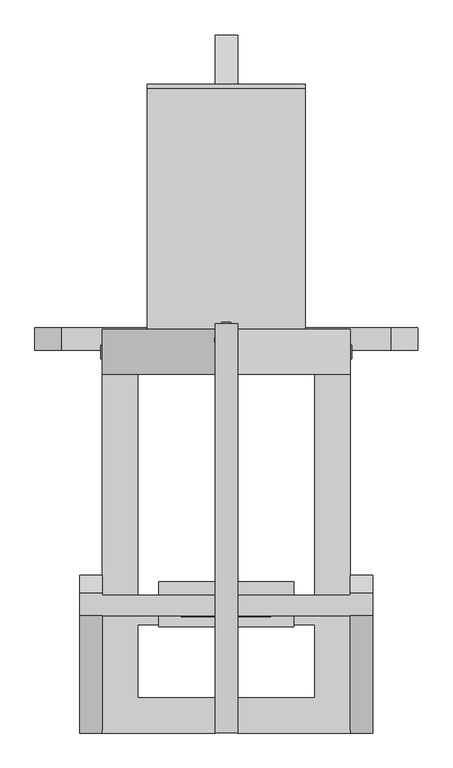
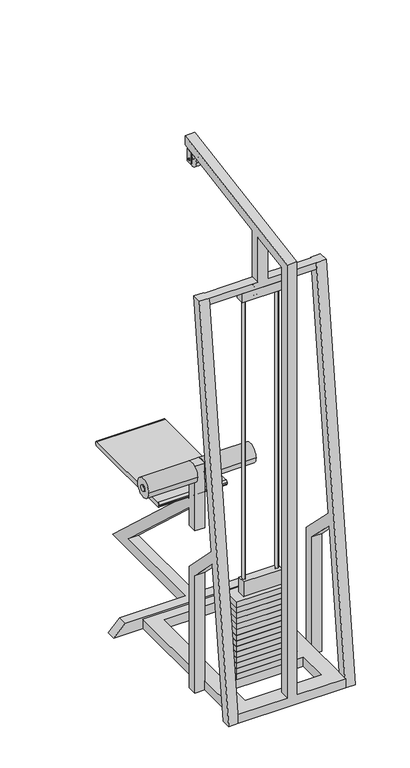
"""IFC4 building model written with IfcOpenShell, lengths in millimetres: proxy geometry."""

from ifc_helpers import new_model, si_unit, point, frame, frame_2d, origin, place, context, project, spatial, polyline, circle_curve, trimmed, segment, composite_curve, outline, extrude, faceted_brep, source, transform, mapped, element, save


def specialty_equipment_45cd0696(model_context):
    return source(origin(), model_context, "Body", "SolidModel", [
        faceted_brep([(130.0819672, 609.7754547, 50.0), (130.0819672, 609.7754547, 0.0), (130.0819672, 109.7754547, 0.0), (130.0819672, 109.7754547, 50.0), (130.0819672, -240.2245453, 0.0), (130.0819672, -240.2245453, 50.0), (130.0819672, -234.1780337, 50.0), (130.0819672, 59.7754547, 0.0), (130.0819672, -189.8602693, 0.0), (130.0819672, -183.8137577, 50.0), (130.0819672, 59.7754547, 50.0), (680.0819672, 609.7754547, 0.0), (680.0819672, 609.7754547, 50.0), (680.0819672, 109.7754547, 50.0), (680.0819672, 109.7754547, 0.0), (680.0819672, -240.2245453, 50.0), (680.0819672, -240.2245453, 0.0), (680.0819672, -234.1780337, 50.0), (680.0819672, 59.7754547, 50.0), (680.0819672, -183.8137577, 50.0), (680.0819672, -189.8602693, 0.0), (680.0819672, 59.7754547, 0.0), (380.0819672, -240.2245453, 50.0), (380.0819672, -190.2245453, 50.0), (430.0819672, -190.2245453, 50.0), (430.0819672, -240.2245453, 50.0), (210.0819672, 559.7754547, 50.0), (600.0819672, 559.7754547, 50.0), (600.0819672, 49.7754547, 50.0), (210.0819672, 49.7754547, 50.0), (210.0819672, -0.2245453, 50.0), (600.0819672, -0.2245453, 50.0), (600.0819672, -160.2245453, 50.0), (210.0819672, -160.2245453, 50.0), (730.0819672, 109.7754547, 0.0), (730.0819672, 59.7754547, 0.0), (730.0819672, -189.8602693, 0.0), (730.0819672, -240.2245453, 0.0), (80.0819672, -240.2245453, 0.0), (80.0819672, -189.8602693, 0.0), (80.0819672, 59.7754547, 0.0), (80.0819672, 109.7754547, 0.0), (600.0819672, 559.7754547, 0.0), (210.0819672, 559.7754547, 0.0), (210.0819672, 49.7754547, 0.0), (600.0819672, 49.7754547, 0.0), (600.0819672, -0.2245453, 0.0), (210.0819672, -0.2245453, 0.0), (210.0819672, -160.2245453, 0.0), (600.0819672, -160.2245453, 0.0), (430.0819672, -240.2245453, 2400.0), (380.0819672, -240.2245453, 2400.0), (380.0819672, 667.995404, 2551.3699916), (380.0819672, 667.995404, 2500.6803038), (380.0819672, 70.1397307, 2401.0376916), (380.0819672, 70.1397307, 2150.0), (380.0819672, 65.9071726, 2150.0), (380.0819672, 19.7754547, 2150.0), (380.0819672, 19.7754547, 2392.6436456), (380.0819672, -190.2245453, 2357.6436456), (430.0819672, -190.2245453, 2357.6436456), (430.0819672, 19.7754547, 2392.6436456), (430.0819672, 19.7754547, 2150.0), (430.0819672, 65.9071726, 2150.0), (430.0819672, 70.1397307, 2150.0), (430.0819672, 70.1397307, 2401.0376916), (430.0819672, 667.995404, 2500.6803038), (430.0819672, 667.995404, 2551.3699916), (130.0819672, 19.7754547, 2150.0), (130.0819672, 19.7754547, 2115.0), (680.0819672, 19.7754547, 2115.0), (680.0819672, 19.7754547, 2150.0), (130.0819672, 65.9071726, 2150.0), (130.0819672, 70.1397307, 2150.0), (80.0819672, 70.1397307, 2150.0), (80.0819672, 19.7754547, 2150.0), (730.0819672, 19.7754547, 2150.0), (730.0819672, 70.1397307, 2150.0), (680.0819672, 70.1397307, 2150.0), (680.0819672, 65.9071726, 2150.0), (680.0819672, 65.9071726, 2115.0), (130.0819672, 65.9071726, 2115.0), (730.0819672, -94.0850882, 791.9870741), (730.0819672, 59.7754547, 638.1265312), (730.0819672, 109.7754547, 658.8372093), (730.0819672, -86.4565503, 855.0692143), (680.0819672, -86.4565503, 855.0692143), (680.0819672, 109.7754547, 658.8372093), (680.0819672, 59.7754547, 638.1265312), (680.0819672, -94.0850882, 791.9870741), (80.0819672, -86.4565503, 855.0692143), (80.0819672, 109.7754547, 658.8372093), (80.0819672, 59.7754547, 638.1265312), (80.0819672, -94.0850882, 791.9870741), (130.0819672, -94.0850882, 791.9870741), (130.0819672, 59.7754547, 638.1265312), (130.0819672, 109.7754547, 658.8372093), (130.0819672, -86.4565503, 855.0692143)], [[[0, 1, 2, 3]], [[4, 5, 6]], [[7, 8, 9, 10]], [[11, 12, 13, 14]], [[15, 16, 17]], [[18, 19, 20, 21]], [[12, 0, 3, 10, 9, 6, 5, 22, 23, 24, 25, 15, 17, 19, 18, 13], [26, 27, 28, 29], [30, 31, 32, 33]], [[1, 0, 12, 11]], [[1, 11, 14, 34, 35, 21, 20, 36, 37, 16, 4, 38, 39, 8, 7, 40, 41, 2], [42, 43, 44, 45], [46, 47, 48, 49]], [[42, 27, 26, 43]], [[27, 42, 45, 28]], [[31, 46, 49, 32]], [[16, 15, 25, 50, 51, 22, 5, 4]], [[43, 26, 29, 44]], [[47, 30, 33, 48]], [[45, 44, 29, 28]], [[47, 46, 31, 30]], [[49, 48, 33, 32]], [[51, 52, 53, 54, 55, 56, 57, 58, 59, 23, 22]], [[60, 61, 62, 63, 64, 65, 66, 67, 50, 25, 24]], [[52, 51, 50, 67]], [[53, 52, 67, 66]], [[59, 58, 61, 60]], [[59, 60, 24, 23]], [[54, 53, 66, 65]], [[55, 54, 65, 64]], [[55, 64, 63, 56]], [[58, 57, 68, 69, 70, 71, 62, 61]], [[68, 57, 56, 72, 73, 74, 75]], [[62, 71, 76, 77, 78, 79, 63]], [[80, 81, 72, 56, 63, 79]], [[81, 80, 70, 69]], [[37, 36, 82, 83, 35, 34, 84, 85, 77, 76]], [[86, 87, 13, 18, 88, 89, 19, 17, 71, 70, 80]], [[78, 80, 79]], [[82, 36, 20, 19, 89]], [[83, 82, 89, 88]], [[35, 83, 88, 18, 21]], [[84, 34, 14, 13, 87]], [[85, 84, 87, 86]], [[77, 85, 86, 80, 78]], [[37, 76, 71, 17, 16]], [[38, 75, 74, 90, 91, 41, 40, 92, 93, 39]], [[73, 72, 81]], [[94, 95, 10, 3, 96, 97, 81, 69, 68, 6, 9]], [[39, 93, 94, 9, 8]], [[93, 92, 95, 94]], [[92, 40, 7, 10, 95]], [[41, 91, 96, 3, 2]], [[91, 90, 97, 96]], [[90, 74, 73, 81, 97]], [[75, 38, 4, 6, 68]]]),
        faceted_brep([(430.0819672, 1309.7754547, 0.0), (430.0819672, 713.9421213, 550.0), (430.0819672, 1109.7754547, 550.0), (430.0819672, 1159.7754547, 600.0), (430.0819672, 631.0595963, 600.0), (430.0819672, 631.0595963, 810.0), (430.0819672, 581.0595963, 810.0), (430.0819672, 581.0595963, 460.0), (430.0819672, 631.0595963, 460.0), (430.0819672, 631.0595963, 558.4615385), (430.0819672, 1171.0595963, 60.0), (430.0819672, 659.7754547, 60.0), (430.0819672, 659.7754547, 0.0), (380.0819672, 1309.7754547, 0.0), (380.0819672, 659.7754547, 0.0), (380.0819672, 659.7754547, 60.0), (380.0819672, 1171.0595963, 60.0), (380.0819672, 631.0595963, 558.4615385), (380.0819672, 631.0595963, 460.0), (380.0819672, 581.0595963, 460.0), (380.0819672, 581.0595963, 810.0), (380.0819672, 631.0595963, 810.0), (380.0819672, 631.0595963, 600.0), (380.0819672, 1159.7754547, 600.0), (380.0819672, 1109.7754547, 550.0), (380.0819672, 713.9421213, 550.0), (40.0819672, 659.7754547, 60.0), (40.0819672, 609.7754547, 60.0), (770.0819672, 609.7754547, 60.0), (770.0819672, 659.7754547, 60.0), (830.0819672, 659.7754547, 0.0), (830.0819672, 609.7754547, 0.0), (80.0819672, 609.7754547, 0.0), (80.0819672, 659.7754547, 0.0), (-19.9180328, 659.7754547, 0.0), (-19.9180328, 609.7754547, 0.0)], [[[0, 1, 2, 3, 4, 5, 6, 7, 8, 9, 10, 11, 12]], [[13, 14, 15, 16, 17, 18, 19, 20, 21, 22, 23, 24, 25]], [[1, 0, 13, 25]], [[2, 1, 25, 24]], [[3, 2, 24, 23]], [[3, 23, 22, 4]], [[16, 10, 9, 17]], [[11, 10, 16, 15, 26, 27, 28, 29]], [[0, 12, 30, 31, 32, 33, 14, 13]], [[33, 34, 26, 15, 14]], [[29, 30, 12, 11]], [[32, 31, 28, 27, 35]], [[34, 33, 32, 35]], [[26, 34, 35, 27]], [[30, 29, 28, 31]], [[21, 20, 6, 5]], [[21, 5, 4, 22]], [[8, 18, 17, 9]], [[19, 18, 8, 7]], [[20, 19, 7, 6]]]),
        extrude(outline(composite_curve([segment(polyline([(1191.0595963, 600.0), (651.0595963, 600.0)]), True, "CONTINUOUS"), segment(trimmed(circle_curve(frame_2d((651.0595963, 610.0)), 10.0), [point((651.0595963, 600.0))], [point((641.0595963, 610.0))], False, "CARTESIAN"), True, "CONTINUOUS"), segment(polyline([(641.0595963, 610.0), (641.0595963, 615.5378202)]), True, "CONTINUOUS"), segment(trimmed(circle_curve(frame_2d((651.0595963, 615.5378202)), 10.0), [point((641.0595963, 615.5378202))], [point((650.5168273, 625.5230794))], False, "CARTESIAN"), True, "CONTINUOUS"), segment(trimmed(circle_curve(frame_2d((921.0595963, -4351.6215395)), 4984.4921454), [point((650.5168273, 625.5230794))], [point((1191.6023652, 625.5230794))], False, "CARTESIAN"), True, "CONTINUOUS"), segment(trimmed(circle_curve(frame_2d((1191.0595963, 615.5378202)), 10.0), [point((1191.6023652, 625.5230794))], [point((1201.0595963, 615.5378202))], False, "CARTESIAN"), True, "CONTINUOUS"), segment(polyline([(1201.0595963, 615.5378202), (1201.0595963, 610.0)]), True, "CONTINUOUS"), segment(trimmed(circle_curve(frame_2d((1191.0595963, 610.0)), 10.0), [point((1201.0595963, 610.0))], [point((1191.0595963, 600.0))], False, "CARTESIAN"), True, "CONTINUOUS")], self_intersect=False)), frame((230.0819672, 0.0, 0.0), z_axis=(1.0, 0.0, 0.0), x_axis=(0.0, 1.0, 0.0)), (0.0, 0.0, 1.0), 350.0),
        extrude(outline(composite_curve([segment(trimmed(circle_curve(frame_2d((606.0595963, 765.0)), 50.0), [point((656.0595963, 765.0))], [point((556.0595963, 765.0))], False, "CARTESIAN"), True, "CONTINUOUS"), segment(trimmed(circle_curve(frame_2d((606.0595963, 765.0)), 50.0), [point((556.0595963, 765.0))], [point((656.0595963, 765.0))], False, "CARTESIAN"), True, "CONTINUOUS")], self_intersect=False), holes=[composite_curve([segment(trimmed(circle_curve(frame_2d((606.0595963, 765.0)), 15.0), [point((621.0595963, 765.0))], [point((591.0595963, 765.0))], True, "CARTESIAN"), True, "CONTINUOUS"), segment(trimmed(circle_curve(frame_2d((606.0595963, 765.0)), 15.0), [point((591.0595963, 765.0))], [point((621.0595963, 765.0))], True, "CARTESIAN"), True, "CONTINUOUS")], self_intersect=False)]), frame((130.0819672, 0.0, 0.0), z_axis=(1.0, 0.0, 0.0), x_axis=(0.0, 1.0, 0.0)), (0.0, 0.0, 1.0), 250.0),
        extrude(outline(composite_curve([segment(trimmed(circle_curve(frame_2d((606.0595963, 765.0)), 50.0), [point((656.0595963, 765.0))], [point((556.0595963, 765.0))], False, "CARTESIAN"), True, "CONTINUOUS"), segment(trimmed(circle_curve(frame_2d((606.0595963, 765.0)), 50.0), [point((556.0595963, 765.0))], [point((656.0595963, 765.0))], False, "CARTESIAN"), True, "CONTINUOUS")], self_intersect=False), holes=[composite_curve([segment(trimmed(circle_curve(frame_2d((606.0595963, 765.0)), 15.0), [point((621.0595963, 765.0))], [point((591.0595963, 765.0))], True, "CARTESIAN"), True, "CONTINUOUS"), segment(trimmed(circle_curve(frame_2d((606.0595963, 765.0)), 15.0), [point((591.0595963, 765.0))], [point((621.0595963, 765.0))], True, "CARTESIAN"), True, "CONTINUOUS")], self_intersect=False)]), frame((430.0819672, 0.0, 0.0), z_axis=(1.0, 0.0, 0.0), x_axis=(0.0, 1.0, 0.0)), (0.0, 0.0, 1.0), 250.0),
        extrude(outline(composite_curve([segment(trimmed(circle_curve(frame_2d((606.0595963, 765.0)), 15.0), [point((621.0595963, 765.0))], [point((591.0595963, 765.0))], False, "CARTESIAN"), True, "CONTINUOUS"), segment(trimmed(circle_curve(frame_2d((606.0595963, 765.0)), 15.0), [point((591.0595963, 765.0))], [point((621.0595963, 765.0))], False, "CARTESIAN"), True, "CONTINUOUS")], self_intersect=False)), frame((126.0819672, 0.0, 0.0), z_axis=(1.0, 0.0, 0.0), x_axis=(0.0, 1.0, 0.0)), (0.0, 0.0, 1.0), 558.0),
        extrude(outline(polyline([(646.8008287, 2427.1478746), (616.8008287, 2427.1478746), (616.8008287, 2492.1478746), (646.8008287, 2497.1478746), (646.8008287, 2427.1478746)])), frame((380.0819672, 0.0, 0.0), z_axis=(1.0, 0.0, 0.0), x_axis=(0.0, 1.0, 0.0)), (0.0, 0.0, 1.0), 5.0),
        extrude(outline(composite_curve([segment(trimmed(circle_curve(frame_2d((631.8008287, 2444.6478746)), 40.0), [point((671.8008287, 2444.6478746))], [point((591.8008287, 2444.6478746))], False, "CARTESIAN"), True, "CONTINUOUS"), segment(trimmed(circle_curve(frame_2d((631.8008287, 2444.6478746)), 40.0), [point((591.8008287, 2444.6478746))], [point((671.8008287, 2444.6478746))], False, "CARTESIAN"), True, "CONTINUOUS")], self_intersect=False), holes=[composite_curve([segment(trimmed(circle_curve(frame_2d((631.8008287, 2444.6478746)), 5.0), [point((636.8008287, 2444.6478746))], [point((626.8008287, 2444.6478746))], True, "CARTESIAN"), True, "CONTINUOUS"), segment(trimmed(circle_curve(frame_2d((631.8008287, 2444.6478746)), 5.0), [point((626.8008287, 2444.6478746))], [point((636.8008287, 2444.6478746))], True, "CARTESIAN"), True, "CONTINUOUS")], self_intersect=False)]), frame((395.0819672, 0.0, 0.0), z_axis=(1.0, 0.0, 0.0), x_axis=(0.0, 1.0, 0.0)), (0.0, 0.0, 1.0), 20.0),
        extrude(outline(composite_curve([segment(trimmed(circle_curve(frame_2d((631.8008287, 2444.6478746)), 5.0), [point((636.8008287, 2444.6478746))], [point((626.8008287, 2444.6478746))], False, "CARTESIAN"), True, "CONTINUOUS"), segment(trimmed(circle_curve(frame_2d((631.8008287, 2444.6478746)), 5.0), [point((626.8008287, 2444.6478746))], [point((636.8008287, 2444.6478746))], False, "CARTESIAN"), True, "CONTINUOUS")], self_intersect=False)), frame((379.0819672, 0.0, 0.0), z_axis=(1.0, 0.0, 0.0), x_axis=(0.0, 1.0, 0.0)), (0.0, 0.0, 1.0), 52.0),
        extrude(outline(polyline([(646.8008287, 2427.1478746), (616.8008287, 2427.1478746), (616.8008287, 2492.1478746), (646.8008287, 2497.1478746), (646.8008287, 2427.1478746)])), frame((425.0819672, 0.0, 0.0), z_axis=(1.0, 0.0, 0.0), x_axis=(0.0, 1.0, 0.0)), (0.0, 0.0, 1.0), 5.0),
        extrude(outline(composite_curve([segment(trimmed(circle_curve(frame_2d((490.0819672, 42.8413136)), 8.0), [point((490.0819672, 34.8413136))], [point((490.0819672, 50.8413136))], False, "CARTESIAN"), True, "CONTINUOUS"), segment(trimmed(circle_curve(frame_2d((490.0819672, 42.8413136)), 8.0), [point((490.0819672, 50.8413136))], [point((490.0819672, 34.8413136))], False, "CARTESIAN"), True, "CONTINUOUS")], self_intersect=False)), frame((0.0, 0.0, 50.0), z_axis=(0.0, 0.0, 1.0), x_axis=(1.0, 0.0, 0.0)), (0.0, 0.0, 1.0), 2065.0),
        extrude(outline(composite_curve([segment(trimmed(circle_curve(frame_2d((320.0819672, 42.8413136)), 8.0), [point((320.0819672, 34.8413136))], [point((320.0819672, 50.8413136))], False, "CARTESIAN"), True, "CONTINUOUS"), segment(trimmed(circle_curve(frame_2d((320.0819672, 42.8413136)), 8.0), [point((320.0819672, 50.8413136))], [point((320.0819672, 34.8413136))], False, "CARTESIAN"), True, "CONTINUOUS")], self_intersect=False)), frame((0.0, 0.0, 50.0), z_axis=(0.0, 0.0, 1.0), x_axis=(1.0, 0.0, 0.0)), (0.0, 0.0, 1.0), 2065.0),
        extrude(outline(polyline([(510.0819672, 19.7754547), (300.0819672, 19.7754547), (300.0819672, 65.9071726), (510.0819672, 65.9071726), (510.0819672, 19.7754547)])), frame((0.0, 0.0, 2065.0), z_axis=(0.0, 0.0, 1.0), x_axis=(1.0, 0.0, 0.0)), (0.0, 0.0, 1.0), 50.0),
        extrude(outline(composite_curve([segment(trimmed(circle_curve(frame_2d((110.9071726, 2062.5)), 40.0), [point((150.9071726, 2062.5))], [point((70.9071726, 2062.5))], False, "CARTESIAN"), True, "CONTINUOUS"), segment(trimmed(circle_curve(frame_2d((110.9071726, 2062.5)), 40.0), [point((70.9071726, 2062.5))], [point((150.9071726, 2062.5))], False, "CARTESIAN"), True, "CONTINUOUS")], self_intersect=False), holes=[composite_curve([segment(trimmed(circle_curve(frame_2d((110.9071726, 2062.5)), 5.0), [point((115.9071726, 2062.5))], [point((105.9071726, 2062.5))], True, "CARTESIAN"), True, "CONTINUOUS"), segment(trimmed(circle_curve(frame_2d((110.9071726, 2062.5)), 5.0), [point((105.9071726, 2062.5))], [point((115.9071726, 2062.5))], True, "CARTESIAN"), True, "CONTINUOUS")], self_intersect=False)]), frame((395.0819672, 0.0, 0.0), z_axis=(1.0, 0.0, 0.0), x_axis=(0.0, 1.0, 0.0)), (0.0, 0.0, 1.0), 20.0),
        extrude(outline(composite_curve([segment(trimmed(circle_curve(frame_2d((110.9071726, 2062.5)), 5.0), [point((115.9071726, 2062.5))], [point((105.9071726, 2062.5))], False, "CARTESIAN"), True, "CONTINUOUS"), segment(trimmed(circle_curve(frame_2d((110.9071726, 2062.5)), 5.0), [point((105.9071726, 2062.5))], [point((115.9071726, 2062.5))], False, "CARTESIAN"), True, "CONTINUOUS")], self_intersect=False)), frame((394.0819672, 0.0, 0.0), z_axis=(1.0, 0.0, 0.0), x_axis=(0.0, 1.0, 0.0)), (0.0, 0.0, 1.0), 22.0),
        extrude(outline(polyline([(555.0819672, -4.0928274), (255.0819672, -4.0928274), (255.0819672, 95.9071726), (555.0819672, 95.9071726), (555.0819672, -4.0928274)])), frame((0.0, 0.0, 50.0), z_axis=(0.0, 0.0, 1.0), x_axis=(1.0, 0.0, 0.0)), (0.0, 0.0, 1.0), 30.0),
        extrude(outline(polyline([(555.0819672, -4.0928274), (255.0819672, -4.0928274), (255.0819672, 95.9071726), (555.0819672, 95.9071726), (555.0819672, -4.0928274)])), frame((0.0, 0.0, 80.0), z_axis=(0.0, 0.0, 1.0), x_axis=(1.0, 0.0, 0.0)), (0.0, 0.0, 1.0), 30.0),
        extrude(outline(polyline([(255.0819672, -4.0928274), (255.0819672, 95.9071726), (555.0819672, 95.9071726), (555.0819672, -4.0928274), (255.0819672, -4.0928274)])), frame((0.0, 0.0, 110.0), z_axis=(0.0, 0.0, 1.0), x_axis=(1.0, 0.0, 0.0)), (0.0, 0.0, 1.0), 30.0),
        extrude(outline(polyline([(255.0819672, -4.0928274), (255.0819672, 95.9071726), (555.0819672, 95.9071726), (555.0819672, -4.0928274), (255.0819672, -4.0928274)])), frame((0.0, 0.0, 140.0), z_axis=(0.0, 0.0, 1.0), x_axis=(1.0, 0.0, 0.0)), (0.0, 0.0, 1.0), 30.0),
        extrude(outline(polyline([(255.0819672, -4.0928274), (255.0819672, 95.9071726), (555.0819672, 95.9071726), (555.0819672, -4.0928274), (255.0819672, -4.0928274)])), frame((0.0, 0.0, 170.0), z_axis=(0.0, 0.0, 1.0), x_axis=(1.0, 0.0, 0.0)), (0.0, 0.0, 1.0), 30.0),
        extrude(outline(polyline([(255.0819672, -4.0928274), (255.0819672, 95.9071726), (555.0819672, 95.9071726), (555.0819672, -4.0928274), (255.0819672, -4.0928274)])), frame((0.0, 0.0, 440.0), z_axis=(0.0, 0.0, 1.0), x_axis=(1.0, 0.0, 0.0)), (0.0, 0.0, 1.0), 30.0),
        extrude(outline(polyline([(255.0819672, -4.0928274), (255.0819672, 95.9071726), (555.0819672, 95.9071726), (555.0819672, -4.0928274), (255.0819672, -4.0928274)])), frame((0.0, 0.0, 200.0), z_axis=(0.0, 0.0, 1.0), x_axis=(1.0, 0.0, 0.0)), (0.0, 0.0, 1.0), 30.0),
        extrude(outline(polyline([(255.0819672, -4.0928274), (255.0819672, 95.9071726), (555.0819672, 95.9071726), (555.0819672, -4.0928274), (255.0819672, -4.0928274)])), frame((0.0, 0.0, 230.0), z_axis=(0.0, 0.0, 1.0), x_axis=(1.0, 0.0, 0.0)), (0.0, 0.0, 1.0), 30.0),
        extrude(outline(polyline([(255.0819672, -4.0928274), (255.0819672, 95.9071726), (555.0819672, 95.9071726), (555.0819672, -4.0928274), (255.0819672, -4.0928274)])), frame((0.0, 0.0, 260.0), z_axis=(0.0, 0.0, 1.0), x_axis=(1.0, 0.0, 0.0)), (0.0, 0.0, 1.0), 30.0),
        extrude(outline(polyline([(255.0819672, -4.0928274), (255.0819672, 95.9071726), (555.0819672, 95.9071726), (555.0819672, -4.0928274), (255.0819672, -4.0928274)])), frame((0.0, 0.0, 290.0), z_axis=(0.0, 0.0, 1.0), x_axis=(1.0, 0.0, 0.0)), (0.0, 0.0, 1.0), 30.0),
        extrude(outline(polyline([(255.0819672, -4.0928274), (255.0819672, 95.9071726), (555.0819672, 95.9071726), (555.0819672, -4.0928274), (255.0819672, -4.0928274)])), frame((0.0, 0.0, 320.0), z_axis=(0.0, 0.0, 1.0), x_axis=(1.0, 0.0, 0.0)), (0.0, 0.0, 1.0), 30.0),
        extrude(outline(polyline([(255.0819672, -4.0928274), (255.0819672, 95.9071726), (555.0819672, 95.9071726), (555.0819672, -4.0928274), (255.0819672, -4.0928274)])), frame((0.0, 0.0, 350.0), z_axis=(0.0, 0.0, 1.0), x_axis=(1.0, 0.0, 0.0)), (0.0, 0.0, 1.0), 30.0),
        extrude(outline(polyline([(255.0819672, -4.0928274), (255.0819672, 95.9071726), (555.0819672, 95.9071726), (555.0819672, -4.0928274), (255.0819672, -4.0928274)])), frame((0.0, 0.0, 380.0), z_axis=(0.0, 0.0, 1.0), x_axis=(1.0, 0.0, 0.0)), (0.0, 0.0, 1.0), 30.0),
        extrude(outline(polyline([(255.0819672, -4.0928274), (255.0819672, 95.9071726), (555.0819672, 95.9071726), (555.0819672, -4.0928274), (255.0819672, -4.0928274)])), frame((0.0, 0.0, 410.0), z_axis=(0.0, 0.0, 1.0), x_axis=(1.0, 0.0, 0.0)), (0.0, 0.0, 1.0), 30.0),
        extrude(outline(polyline([(305.0819672, 17.9504864), (305.0819672, 59.7754547), (503.8290161, 59.7754547), (503.8290161, 17.9504864), (305.0819672, 17.9504864)])), frame((0.0, 0.0, 470.0), z_axis=(0.0, 0.0, 1.0), x_axis=(1.0, 0.0, 0.0)), (0.0, 0.0, 1.0), 80.0),
    ])


if __name__ == "__main__":
    model = new_model("IFC4")
    model_context = context("Model", 3, world=origin())
    ifc_project = project(units=[si_unit("LENGTHUNIT", "METRE", prefix="MILLI")], contexts=[model_context])
    site = spatial("IfcSite", under=ifc_project)
    building = spatial("IfcBuilding", under=site)
    placement = place(None, origin())
    specialty_equipment_shape = specialty_equipment_45cd0696(model_context)
    element("IfcBuildingElementProxy", 1, Name="Specialty Equipment", at=placement, inside=building, context=model_context, shape_type="MappedRepresentation", body=[
        mapped(specialty_equipment_shape, transform((0.0, 0.0, 0.0), x_axis=(1.0, 0.0, 0.0), y_axis=(0.0, 1.0, 0.0), z_axis=(0.0, 0.0, 1.0))),
    ])
    save(model, "model.ifc")

# Revit data of these elements
# Type
#   Assembly Code = "E1090"
#   Top width = 1' - 0.07125"
#   Height = 10' - 9.92126"
#   Frame thickness = 0' - 1.9685"
#   vinyl = Plastic - Black
#   Metal Material = Metal - painted
#   Metal - painted = Metal - painted
#   Black = none
#   Default Elevation = 0
# Element 1 (IfcBuildingElementProxy)
#   Materials on its faces: "Metal - painted", "Plastic - Black"
# Materials
#   "Plastic - Black": colour RGB 0 0 0, transparency 0
#   "Metal - painted": colour RGB 247 247 239, transparency 0
